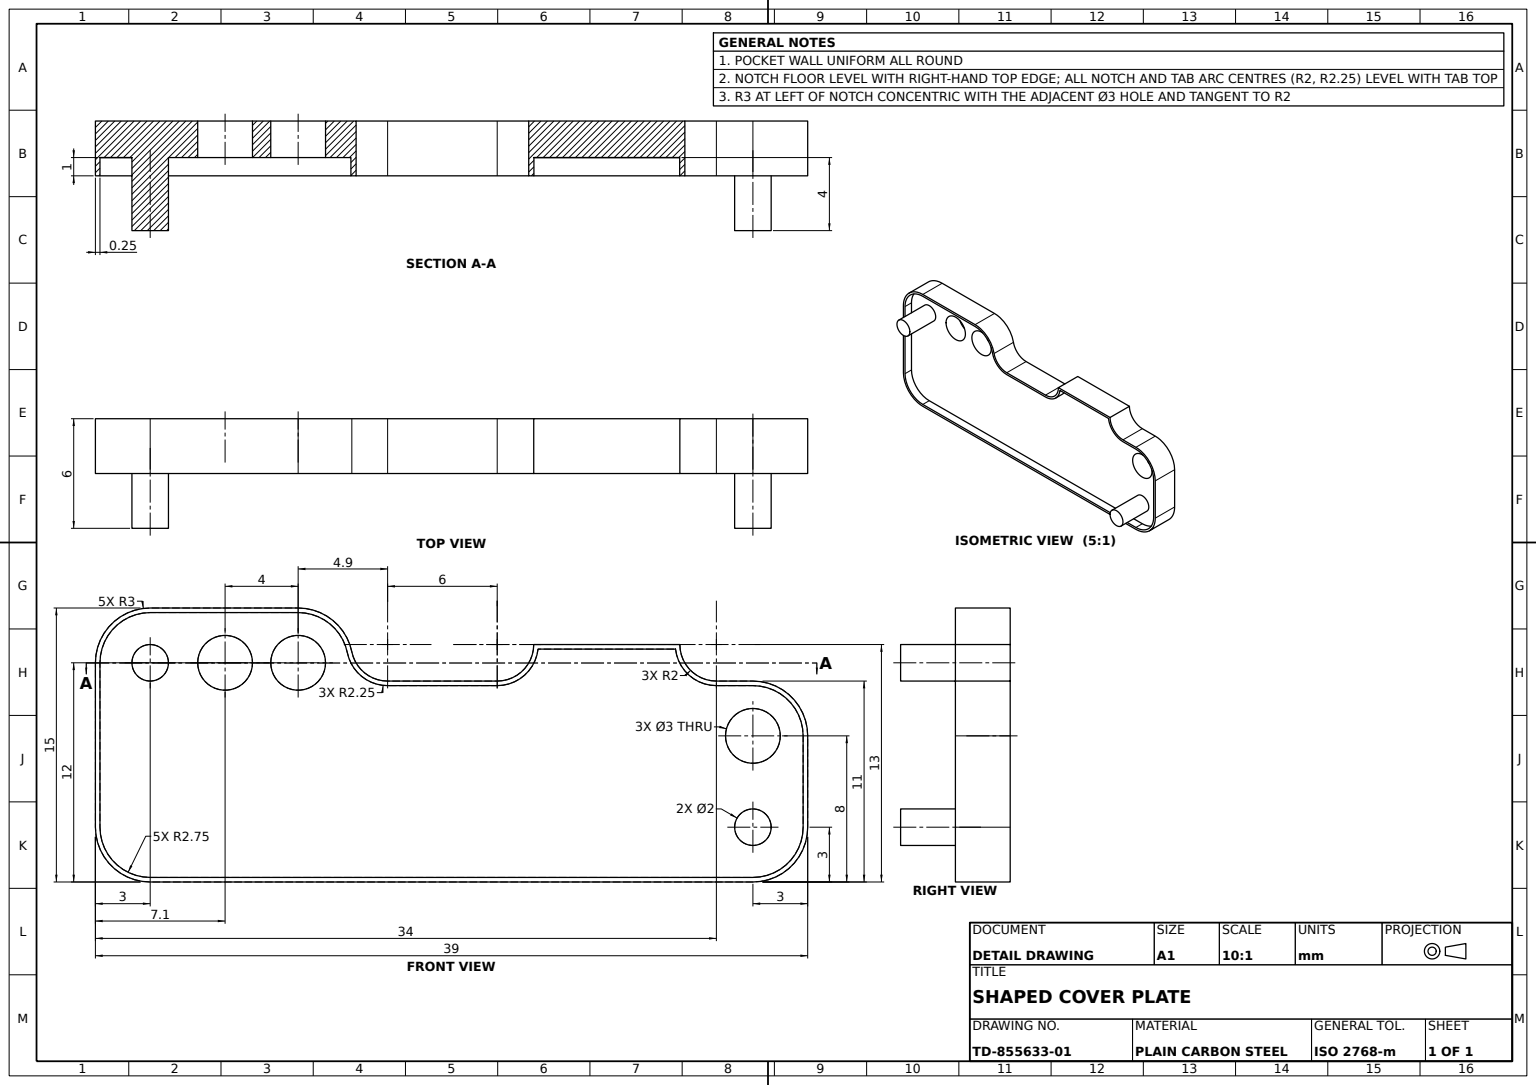
SolidWorks part; units mm, degrees
material "Plain Carbon Steel"
ref_plane "Front Plane" through (0, 0, 0) normal (0, 0, 1) x (1, 0, 0)
ref_plane "Top Plane" through (0, 0, 0) normal (0, 1, 0) x (1, 0, 0)
ref_plane "Right Plane" through (0, 0, 0) normal (1, 0, 0) x (0, 0, -1)
sketch "Base Plate Sketch" plane through (0, 0, 0) normal (0, 0, 1) x (1, 0, 0)
  line L0 (0, 3) -> (0, 12)
  line L1 (3, 0) -> (36, 0)
  line L2 (39, 3) -> (39, 8)
  line L3 (36, 11) -> (34, 11)
  line L5 (32, 13) -> (24, 13)
  line L7 (22, 11) -> (16, 11)
  line L9 (11.101, 15) -> (3, 15)
  arc A0 (39, 8) -> (36, 11) centre (36, 8) ccw
  arc A1 (36, 0) -> (39, 3) centre (36, 3) ccw
  arc A2 (0, 3) -> (3, 0) centre (3, 3) ccw
  arc A3 (0, 12) -> (3, 15) centre (3, 12) cw
  arc A4 (16, 11) -> (14.0404, 12.6) centre (16, 13) cw
  arc A5 (14.0404, 12.6) -> (11.101, 15) centre (11.101, 12) ccw
  arc A6 (22, 11) -> (24, 13) centre (22, 13) ccw
  arc A7 (32, 13) -> (34, 11) centre (34, 13) ccw
  point P17 (0, 0)
  dimension "D1" = 3
  dimension "D2" = 2
  dimension "D3" = 3
  dimension "D10" = 34
  dimension "D6" = 2
  dimension "D11" = 2
  dimension "D4" = 39
  dimension "D5" = 5
  dimension "D7" = 8
  dimension "D8" = 13
  dimension "D9" = 11
  dimension "D12" = 6
  dimension "D13" = 4.899
extrude "Base Plate" add sketch "Base Plate Sketch" along normal blind 2
sketch "Perimeter Rim Sketch" plane through (0, 0, 2) normal (0, 0, 1) x (1, 0, 0)
  line L0 (31.7639, 12.75) -> (24.2361, 12.75)
  line L1 (22, 10.75) -> (16, 10.75)
  line L2 (11.101, 14.75) -> (3, 14.75)
  line L3 (0.25, 12) -> (0.25, 3)
  line L4 (3, 0.25) -> (36, 0.25)
  line L5 (38.75, 3) -> (38.75, 8)
  line L6 (36, 10.75) -> (34, 10.75)
  line L7 (32, 13) -> (24, 13)
  line L8 (22, 11) -> (16, 11)
  line L9 (11.101, 15) -> (3, 15)
  line L10 (0, 12) -> (0, 3)
  line L11 (3, 0) -> (36, 0)
  line L12 (39, 3) -> (39, 8)
  line L13 (36, 11) -> (34, 11)
  line L14 (32, 13) -> (24, 13)
  line L15 (22, 11) -> (16, 11)
  line L16 (11.101, 15) -> (3, 15)
  line L17 (0, 12) -> (0, 3)
  line L18 (3, 0) -> (36, 0)
  line L19 (39, 3) -> (39, 8)
  line L20 (36, 11) -> (34, 11)
  arc A0 (22, 10.75) -> (24.2361, 12.75) centre (22, 13) ccw
  arc A1 (13.7955, 12.55) -> (16, 10.75) centre (16, 13) ccw
  arc A2 (13.7955, 12.55) -> (11.101, 14.75) centre (11.101, 12) ccw
  arc A3 (3, 14.75) -> (0.25, 12) centre (3, 12) ccw
  arc A4 (0.25, 3) -> (3, 0.25) centre (3, 3) ccw
  arc A5 (36, 0.25) -> (38.75, 3) centre (36, 3) ccw
  arc A6 (38.75, 8) -> (36, 10.75) centre (36, 8) ccw
  arc A7 (31.7639, 12.75) -> (34, 10.75) centre (34, 13) ccw
  arc A8 (32, 13) -> (34, 11) centre (34, 13) ccw
  arc A9 (22, 11) -> (24, 13) centre (22, 13) ccw
  arc A10 (14.0404, 12.6) -> (16, 11) centre (16, 13) ccw
  arc A11 (14.0404, 12.6) -> (11.101, 15) centre (11.101, 12) ccw
  arc A12 (3, 15) -> (0, 12) centre (3, 12) ccw
  arc A13 (0, 3) -> (3, 0) centre (3, 3) ccw
  arc A14 (36, 0) -> (39, 3) centre (36, 3) ccw
  arc A15 (39, 8) -> (36, 11) centre (36, 8) ccw
  arc A16 (32, 13) -> (34, 11) centre (34, 13) ccw
  arc A17 (22, 11) -> (24, 13) centre (22, 13) ccw
  arc A18 (14.0404, 12.6) -> (16, 11) centre (16, 13) ccw
  arc A19 (14.0404, 12.6) -> (11.101, 15) centre (11.101, 12) ccw
  arc A20 (3, 15) -> (0, 12) centre (3, 12) ccw
  arc A21 (0, 3) -> (3, 0) centre (3, 3) ccw
  arc A22 (36, 0) -> (39, 3) centre (36, 3) ccw
  arc A23 (39, 8) -> (36, 11) centre (36, 8) ccw
  dimension "D1" = 0
  dimension "D2" = 0.25
extrude "Perimeter Rim" add sketch "Perimeter Rim Sketch" along normal blind 1
sketch "Pin 1 Sketch" plane through (0, 0, 2) normal (0, 0, 1) x (1, 0, 0)
  circle A0 centre (36, 3) radius 1
  dimension "D1" = 2
extrude "Pin 1 Ø2" add sketch "Pin 1 Sketch" along normal blind 4
sketch "Pin 2 Sketch" plane through (0, 0, 2) normal (0, 0, 1) x (1, 0, 0)
  circle A0 centre (3, 12) radius 1
  dimension "D1" = 2
extrude "Pin 2 Ø2" add sketch "Pin 2 Sketch" along normal blind 4
sketch "Through Holes Sketch" plane through (0, 0, 2) normal (0, 0, 1) x (1, 0, 0)
  circle A0 centre (36, 8) radius 1.5
  circle A1 centre (11.101, 12) radius 1.5
  circle A2 centre (7.101, 12) radius 1.5
  dimension "D1" = 3
  dimension "D2" = 3
  dimension "D3" = 3
  dimension "D4" = 12
  dimension "D5" = 7.101
extrude "Through Holes 3xØ3" cut sketch "Through Holes Sketch" against normal blind 4
